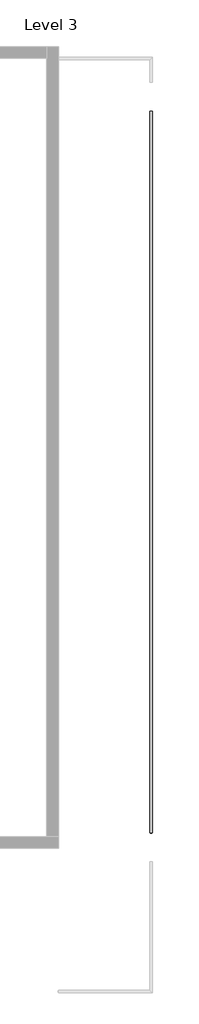
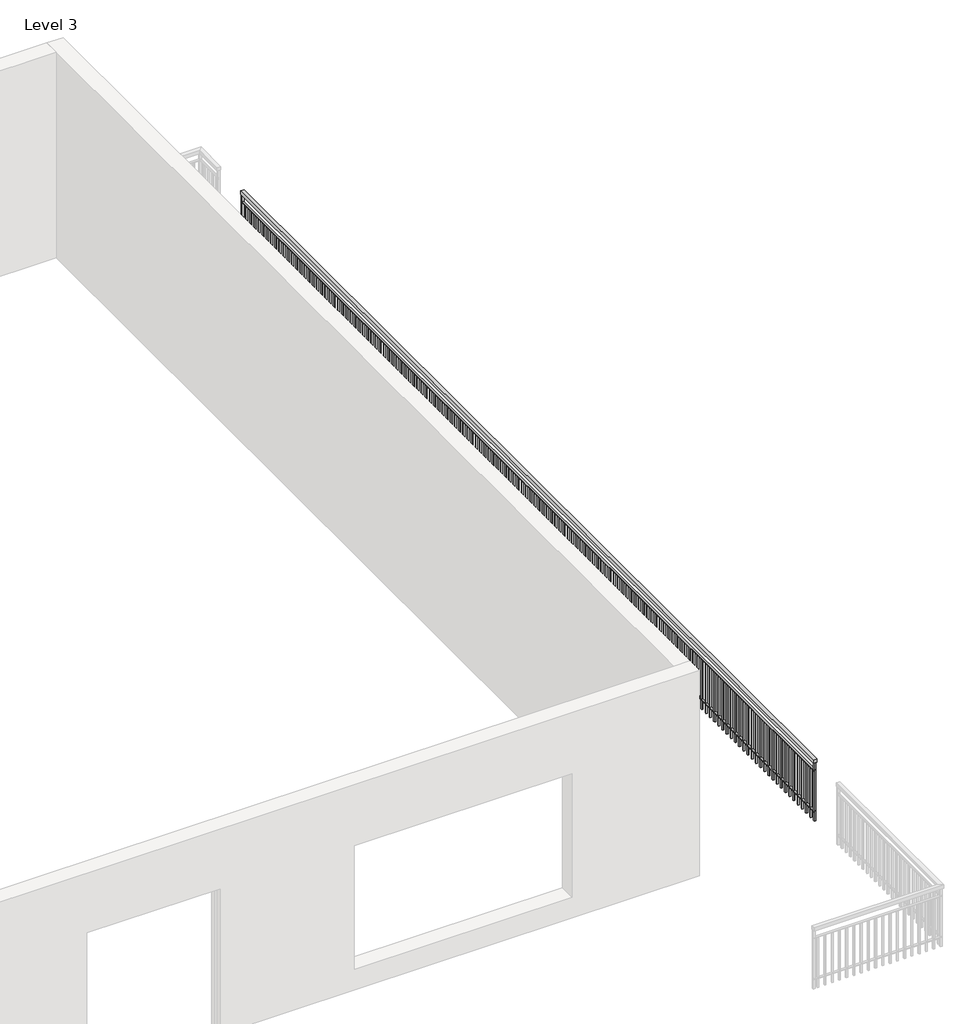
# One storey, part 3 of 4: 1 railing.
"""IFC4 building model written with IfcOpenShell, lengths in millimetres."""

from ifc_helpers import new_model, si_unit, point, frame, frame_2d, origin, place, context, project, spatial, polyline, circle_curve, trimmed, segment, composite_curve, outline, extrude, element, save

model = new_model("IFC4")

# Units and contexts
model_context = context("Model", 3, world=origin())
ifc_project = project(units=[si_unit("LENGTHUNIT", "METRE", prefix="MILLI")], contexts=[model_context])

# Site, building, storey
site = spatial("IfcSite", under=ifc_project)
building = spatial("IfcBuilding", under=site)
storey = spatial("IfcBuildingStorey", under=building, Name="Level 3", Elevation=3810.0)

# Railing
placement = place(None, origin())
element("IfcRailing", 1, ObjectType="Handrail - Rectangular", at=placement, inside=storey, context=model_context, shape_type="SweptSolid", body=[
    extrude(outline(polyline([(8462.6425759, 8145.5475503), (8513.4425759, 8145.5475503), (8513.4425759, -5773.6524497), (8462.6425759, -5773.6524497), (8462.6425759, 8145.5475503)])), frame((0.0, 0.0, 4673.6), z_axis=(0.0, 0.0, 1.0), x_axis=(1.0, 0.0, 0.0)), (0.0, 0.0, 1.0), 50.8),
    extrude(outline(composite_curve([segment(trimmed(circle_curve(frame_2d((4559.3, 8488.0425759)), 12.7), [point((4559.3, 8500.7425759))], [point((4559.3, 8475.3425759))], False, "CARTESIAN"), True, "CONTINUOUS"), segment(trimmed(circle_curve(frame_2d((4559.3, 8488.0425759)), 12.7), [point((4559.3, 8475.3425759))], [point((4559.3, 8500.7425759))], False, "CARTESIAN"), True, "CONTINUOUS")], self_intersect=False)), frame((0.0, -5773.6524497, 0.0), z_axis=(0.0, 1.0, 0.0), x_axis=(0.0, 0.0, 1.0)), (0.0, 0.0, 1.0), 13919.2),
    extrude(outline(composite_curve([segment(trimmed(circle_curve(frame_2d((3949.7, 8488.0425759)), 12.7), [point((3949.7, 8500.7425759))], [point((3949.7, 8475.3425759))], False, "CARTESIAN"), True, "CONTINUOUS"), segment(trimmed(circle_curve(frame_2d((3949.7, 8488.0425759)), 12.7), [point((3949.7, 8475.3425759))], [point((3949.7, 8500.7425759))], False, "CARTESIAN"), True, "CONTINUOUS")], self_intersect=False)), frame((0.0, -5773.6524497, 0.0), z_axis=(0.0, 1.0, 0.0), x_axis=(0.0, 0.0, 1.0)), (0.0, 0.0, 1.0), 13919.2),
    extrude(outline(polyline([(8478.5175759, -5662.5274497), (8497.5675759, -5662.5274497), (8497.5675759, -5681.5774497), (8478.5175759, -5681.5774497), (8478.5175759, -5662.5274497)])), frame((0.0, 0.0, 3810.0), z_axis=(0.0, 0.0, 1.0), x_axis=(1.0, 0.0, 0.0)), (0.0, 0.0, 1.0), 736.6),
    extrude(outline(polyline([(8478.5175759, -5560.9274497), (8497.5675759, -5560.9274497), (8497.5675759, -5579.9774497), (8478.5175759, -5579.9774497), (8478.5175759, -5560.9274497)])), frame((0.0, 0.0, 3810.0), z_axis=(0.0, 0.0, 1.0), x_axis=(1.0, 0.0, 0.0)), (0.0, 0.0, 1.0), 736.6),
    extrude(outline(polyline([(8478.5175759, -5459.3274497), (8497.5675759, -5459.3274497), (8497.5675759, -5478.3774497), (8478.5175759, -5478.3774497), (8478.5175759, -5459.3274497)])), frame((0.0, 0.0, 3810.0), z_axis=(0.0, 0.0, 1.0), x_axis=(1.0, 0.0, 0.0)), (0.0, 0.0, 1.0), 736.6),
    extrude(outline(polyline([(8478.5175759, -5357.7274497), (8497.5675759, -5357.7274497), (8497.5675759, -5376.7774497), (8478.5175759, -5376.7774497), (8478.5175759, -5357.7274497)])), frame((0.0, 0.0, 3810.0), z_axis=(0.0, 0.0, 1.0), x_axis=(1.0, 0.0, 0.0)), (0.0, 0.0, 1.0), 736.6),
    extrude(outline(polyline([(8478.5175759, -5256.1274497), (8497.5675759, -5256.1274497), (8497.5675759, -5275.1774497), (8478.5175759, -5275.1774497), (8478.5175759, -5256.1274497)])), frame((0.0, 0.0, 3810.0), z_axis=(0.0, 0.0, 1.0), x_axis=(1.0, 0.0, 0.0)), (0.0, 0.0, 1.0), 736.6),
    extrude(outline(polyline([(8478.5175759, -5154.5274497), (8497.5675759, -5154.5274497), (8497.5675759, -5173.5774497), (8478.5175759, -5173.5774497), (8478.5175759, -5154.5274497)])), frame((0.0, 0.0, 3810.0), z_axis=(0.0, 0.0, 1.0), x_axis=(1.0, 0.0, 0.0)), (0.0, 0.0, 1.0), 736.6),
    extrude(outline(polyline([(8478.5175759, -5052.9274497), (8497.5675759, -5052.9274497), (8497.5675759, -5071.9774497), (8478.5175759, -5071.9774497), (8478.5175759, -5052.9274497)])), frame((0.0, 0.0, 3810.0), z_axis=(0.0, 0.0, 1.0), x_axis=(1.0, 0.0, 0.0)), (0.0, 0.0, 1.0), 736.6),
    extrude(outline(polyline([(8478.5175759, -4951.3274497), (8497.5675759, -4951.3274497), (8497.5675759, -4970.3774497), (8478.5175759, -4970.3774497), (8478.5175759, -4951.3274497)])), frame((0.0, 0.0, 3810.0), z_axis=(0.0, 0.0, 1.0), x_axis=(1.0, 0.0, 0.0)), (0.0, 0.0, 1.0), 736.6),
    extrude(outline(polyline([(8478.5175759, -4849.7274497), (8497.5675759, -4849.7274497), (8497.5675759, -4868.7774497), (8478.5175759, -4868.7774497), (8478.5175759, -4849.7274497)])), frame((0.0, 0.0, 3810.0), z_axis=(0.0, 0.0, 1.0), x_axis=(1.0, 0.0, 0.0)), (0.0, 0.0, 1.0), 736.6),
    extrude(outline(polyline([(8478.5175759, -4748.1274497), (8497.5675759, -4748.1274497), (8497.5675759, -4767.1774497), (8478.5175759, -4767.1774497), (8478.5175759, -4748.1274497)])), frame((0.0, 0.0, 3810.0), z_axis=(0.0, 0.0, 1.0), x_axis=(1.0, 0.0, 0.0)), (0.0, 0.0, 1.0), 736.6),
    extrude(outline(polyline([(8478.5175759, -4646.5274497), (8497.5675759, -4646.5274497), (8497.5675759, -4665.5774497), (8478.5175759, -4665.5774497), (8478.5175759, -4646.5274497)])), frame((0.0, 0.0, 3810.0), z_axis=(0.0, 0.0, 1.0), x_axis=(1.0, 0.0, 0.0)), (0.0, 0.0, 1.0), 736.6),
    extrude(outline(polyline([(8478.5175759, -4544.9274497), (8497.5675759, -4544.9274497), (8497.5675759, -4563.9774497), (8478.5175759, -4563.9774497), (8478.5175759, -4544.9274497)])), frame((0.0, 0.0, 3810.0), z_axis=(0.0, 0.0, 1.0), x_axis=(1.0, 0.0, 0.0)), (0.0, 0.0, 1.0), 736.6),
    extrude(outline(polyline([(8478.5175759, -4443.3274497), (8497.5675759, -4443.3274497), (8497.5675759, -4462.3774497), (8478.5175759, -4462.3774497), (8478.5175759, -4443.3274497)])), frame((0.0, 0.0, 3810.0), z_axis=(0.0, 0.0, 1.0), x_axis=(1.0, 0.0, 0.0)), (0.0, 0.0, 1.0), 736.6),
    extrude(outline(polyline([(8478.5175759, -4341.7274497), (8497.5675759, -4341.7274497), (8497.5675759, -4360.7774497), (8478.5175759, -4360.7774497), (8478.5175759, -4341.7274497)])), frame((0.0, 0.0, 3810.0), z_axis=(0.0, 0.0, 1.0), x_axis=(1.0, 0.0, 0.0)), (0.0, 0.0, 1.0), 736.6),
    extrude(outline(polyline([(8478.5175759, -4240.1274497), (8497.5675759, -4240.1274497), (8497.5675759, -4259.1774497), (8478.5175759, -4259.1774497), (8478.5175759, -4240.1274497)])), frame((0.0, 0.0, 3810.0), z_axis=(0.0, 0.0, 1.0), x_axis=(1.0, 0.0, 0.0)), (0.0, 0.0, 1.0), 736.6),
    extrude(outline(polyline([(8478.5175759, -4138.5274497), (8497.5675759, -4138.5274497), (8497.5675759, -4157.5774497), (8478.5175759, -4157.5774497), (8478.5175759, -4138.5274497)])), frame((0.0, 0.0, 3810.0), z_axis=(0.0, 0.0, 1.0), x_axis=(1.0, 0.0, 0.0)), (0.0, 0.0, 1.0), 736.6),
    extrude(outline(polyline([(8478.5175759, -4036.9274497), (8497.5675759, -4036.9274497), (8497.5675759, -4055.9774497), (8478.5175759, -4055.9774497), (8478.5175759, -4036.9274497)])), frame((0.0, 0.0, 3810.0), z_axis=(0.0, 0.0, 1.0), x_axis=(1.0, 0.0, 0.0)), (0.0, 0.0, 1.0), 736.6),
    extrude(outline(polyline([(8478.5175759, -3935.3274497), (8497.5675759, -3935.3274497), (8497.5675759, -3954.3774497), (8478.5175759, -3954.3774497), (8478.5175759, -3935.3274497)])), frame((0.0, 0.0, 3810.0), z_axis=(0.0, 0.0, 1.0), x_axis=(1.0, 0.0, 0.0)), (0.0, 0.0, 1.0), 736.6),
    extrude(outline(polyline([(8478.5175759, -3833.7274497), (8497.5675759, -3833.7274497), (8497.5675759, -3852.7774497), (8478.5175759, -3852.7774497), (8478.5175759, -3833.7274497)])), frame((0.0, 0.0, 3810.0), z_axis=(0.0, 0.0, 1.0), x_axis=(1.0, 0.0, 0.0)), (0.0, 0.0, 1.0), 736.6),
    extrude(outline(polyline([(8478.5175759, -3732.1274497), (8497.5675759, -3732.1274497), (8497.5675759, -3751.1774497), (8478.5175759, -3751.1774497), (8478.5175759, -3732.1274497)])), frame((0.0, 0.0, 3810.0), z_axis=(0.0, 0.0, 1.0), x_axis=(1.0, 0.0, 0.0)), (0.0, 0.0, 1.0), 736.6),
    extrude(outline(polyline([(8478.5175759, -3630.5274497), (8497.5675759, -3630.5274497), (8497.5675759, -3649.5774497), (8478.5175759, -3649.5774497), (8478.5175759, -3630.5274497)])), frame((0.0, 0.0, 3810.0), z_axis=(0.0, 0.0, 1.0), x_axis=(1.0, 0.0, 0.0)), (0.0, 0.0, 1.0), 736.6),
    extrude(outline(polyline([(8478.5175759, -3528.9274497), (8497.5675759, -3528.9274497), (8497.5675759, -3547.9774497), (8478.5175759, -3547.9774497), (8478.5175759, -3528.9274497)])), frame((0.0, 0.0, 3810.0), z_axis=(0.0, 0.0, 1.0), x_axis=(1.0, 0.0, 0.0)), (0.0, 0.0, 1.0), 736.6),
    extrude(outline(polyline([(8478.5175759, -3427.3274497), (8497.5675759, -3427.3274497), (8497.5675759, -3446.3774497), (8478.5175759, -3446.3774497), (8478.5175759, -3427.3274497)])), frame((0.0, 0.0, 3810.0), z_axis=(0.0, 0.0, 1.0), x_axis=(1.0, 0.0, 0.0)), (0.0, 0.0, 1.0), 736.6),
    extrude(outline(polyline([(8478.5175759, -3325.7274497), (8497.5675759, -3325.7274497), (8497.5675759, -3344.7774497), (8478.5175759, -3344.7774497), (8478.5175759, -3325.7274497)])), frame((0.0, 0.0, 3810.0), z_axis=(0.0, 0.0, 1.0), x_axis=(1.0, 0.0, 0.0)), (0.0, 0.0, 1.0), 736.6),
    extrude(outline(polyline([(8478.5175759, -3224.1274497), (8497.5675759, -3224.1274497), (8497.5675759, -3243.1774497), (8478.5175759, -3243.1774497), (8478.5175759, -3224.1274497)])), frame((0.0, 0.0, 3810.0), z_axis=(0.0, 0.0, 1.0), x_axis=(1.0, 0.0, 0.0)), (0.0, 0.0, 1.0), 736.6),
    extrude(outline(polyline([(8478.5175759, -3122.5274497), (8497.5675759, -3122.5274497), (8497.5675759, -3141.5774497), (8478.5175759, -3141.5774497), (8478.5175759, -3122.5274497)])), frame((0.0, 0.0, 3810.0), z_axis=(0.0, 0.0, 1.0), x_axis=(1.0, 0.0, 0.0)), (0.0, 0.0, 1.0), 736.6),
    extrude(outline(polyline([(8478.5175759, -3020.9274497), (8497.5675759, -3020.9274497), (8497.5675759, -3039.9774497), (8478.5175759, -3039.9774497), (8478.5175759, -3020.9274497)])), frame((0.0, 0.0, 3810.0), z_axis=(0.0, 0.0, 1.0), x_axis=(1.0, 0.0, 0.0)), (0.0, 0.0, 1.0), 736.6),
    extrude(outline(polyline([(8478.5175759, -2919.3274497), (8497.5675759, -2919.3274497), (8497.5675759, -2938.3774497), (8478.5175759, -2938.3774497), (8478.5175759, -2919.3274497)])), frame((0.0, 0.0, 3810.0), z_axis=(0.0, 0.0, 1.0), x_axis=(1.0, 0.0, 0.0)), (0.0, 0.0, 1.0), 736.6),
    extrude(outline(polyline([(8478.5175759, -2817.7274497), (8497.5675759, -2817.7274497), (8497.5675759, -2836.7774497), (8478.5175759, -2836.7774497), (8478.5175759, -2817.7274497)])), frame((0.0, 0.0, 3810.0), z_axis=(0.0, 0.0, 1.0), x_axis=(1.0, 0.0, 0.0)), (0.0, 0.0, 1.0), 736.6),
    extrude(outline(polyline([(8478.5175759, -2716.1274497), (8497.5675759, -2716.1274497), (8497.5675759, -2735.1774497), (8478.5175759, -2735.1774497), (8478.5175759, -2716.1274497)])), frame((0.0, 0.0, 3810.0), z_axis=(0.0, 0.0, 1.0), x_axis=(1.0, 0.0, 0.0)), (0.0, 0.0, 1.0), 736.6),
    extrude(outline(polyline([(8478.5175759, -2614.5274497), (8497.5675759, -2614.5274497), (8497.5675759, -2633.5774497), (8478.5175759, -2633.5774497), (8478.5175759, -2614.5274497)])), frame((0.0, 0.0, 3810.0), z_axis=(0.0, 0.0, 1.0), x_axis=(1.0, 0.0, 0.0)), (0.0, 0.0, 1.0), 736.6),
    extrude(outline(polyline([(8478.5175759, -2512.9274497), (8497.5675759, -2512.9274497), (8497.5675759, -2531.9774497), (8478.5175759, -2531.9774497), (8478.5175759, -2512.9274497)])), frame((0.0, 0.0, 3810.0), z_axis=(0.0, 0.0, 1.0), x_axis=(1.0, 0.0, 0.0)), (0.0, 0.0, 1.0), 736.6),
    extrude(outline(polyline([(8478.5175759, -2411.3274497), (8497.5675759, -2411.3274497), (8497.5675759, -2430.3774497), (8478.5175759, -2430.3774497), (8478.5175759, -2411.3274497)])), frame((0.0, 0.0, 3810.0), z_axis=(0.0, 0.0, 1.0), x_axis=(1.0, 0.0, 0.0)), (0.0, 0.0, 1.0), 736.6),
    extrude(outline(polyline([(8478.5175759, -2309.7274497), (8497.5675759, -2309.7274497), (8497.5675759, -2328.7774497), (8478.5175759, -2328.7774497), (8478.5175759, -2309.7274497)])), frame((0.0, 0.0, 3810.0), z_axis=(0.0, 0.0, 1.0), x_axis=(1.0, 0.0, 0.0)), (0.0, 0.0, 1.0), 736.6),
    extrude(outline(polyline([(8478.5175759, -2208.1274497), (8497.5675759, -2208.1274497), (8497.5675759, -2227.1774497), (8478.5175759, -2227.1774497), (8478.5175759, -2208.1274497)])), frame((0.0, 0.0, 3810.0), z_axis=(0.0, 0.0, 1.0), x_axis=(1.0, 0.0, 0.0)), (0.0, 0.0, 1.0), 736.6),
    extrude(outline(polyline([(8478.5175759, -2106.5274497), (8497.5675759, -2106.5274497), (8497.5675759, -2125.5774497), (8478.5175759, -2125.5774497), (8478.5175759, -2106.5274497)])), frame((0.0, 0.0, 3810.0), z_axis=(0.0, 0.0, 1.0), x_axis=(1.0, 0.0, 0.0)), (0.0, 0.0, 1.0), 736.6),
    extrude(outline(polyline([(8478.5175759, -2004.9274497), (8497.5675759, -2004.9274497), (8497.5675759, -2023.9774497), (8478.5175759, -2023.9774497), (8478.5175759, -2004.9274497)])), frame((0.0, 0.0, 3810.0), z_axis=(0.0, 0.0, 1.0), x_axis=(1.0, 0.0, 0.0)), (0.0, 0.0, 1.0), 736.6),
    extrude(outline(polyline([(8478.5175759, -1903.3274497), (8497.5675759, -1903.3274497), (8497.5675759, -1922.3774497), (8478.5175759, -1922.3774497), (8478.5175759, -1903.3274497)])), frame((0.0, 0.0, 3810.0), z_axis=(0.0, 0.0, 1.0), x_axis=(1.0, 0.0, 0.0)), (0.0, 0.0, 1.0), 736.6),
    extrude(outline(polyline([(8478.5175759, -1801.7274497), (8497.5675759, -1801.7274497), (8497.5675759, -1820.7774497), (8478.5175759, -1820.7774497), (8478.5175759, -1801.7274497)])), frame((0.0, 0.0, 3810.0), z_axis=(0.0, 0.0, 1.0), x_axis=(1.0, 0.0, 0.0)), (0.0, 0.0, 1.0), 736.6),
    extrude(outline(polyline([(8478.5175759, -1700.1274497), (8497.5675759, -1700.1274497), (8497.5675759, -1719.1774497), (8478.5175759, -1719.1774497), (8478.5175759, -1700.1274497)])), frame((0.0, 0.0, 3810.0), z_axis=(0.0, 0.0, 1.0), x_axis=(1.0, 0.0, 0.0)), (0.0, 0.0, 1.0), 736.6),
    extrude(outline(polyline([(8478.5175759, -1598.5274497), (8497.5675759, -1598.5274497), (8497.5675759, -1617.5774497), (8478.5175759, -1617.5774497), (8478.5175759, -1598.5274497)])), frame((0.0, 0.0, 3810.0), z_axis=(0.0, 0.0, 1.0), x_axis=(1.0, 0.0, 0.0)), (0.0, 0.0, 1.0), 736.6),
    extrude(outline(polyline([(8478.5175759, -1496.9274497), (8497.5675759, -1496.9274497), (8497.5675759, -1515.9774497), (8478.5175759, -1515.9774497), (8478.5175759, -1496.9274497)])), frame((0.0, 0.0, 3810.0), z_axis=(0.0, 0.0, 1.0), x_axis=(1.0, 0.0, 0.0)), (0.0, 0.0, 1.0), 736.6),
    extrude(outline(polyline([(8478.5175759, -1395.3274497), (8497.5675759, -1395.3274497), (8497.5675759, -1414.3774497), (8478.5175759, -1414.3774497), (8478.5175759, -1395.3274497)])), frame((0.0, 0.0, 3810.0), z_axis=(0.0, 0.0, 1.0), x_axis=(1.0, 0.0, 0.0)), (0.0, 0.0, 1.0), 736.6),
    extrude(outline(polyline([(8478.5175759, -1293.7274497), (8497.5675759, -1293.7274497), (8497.5675759, -1312.7774497), (8478.5175759, -1312.7774497), (8478.5175759, -1293.7274497)])), frame((0.0, 0.0, 3810.0), z_axis=(0.0, 0.0, 1.0), x_axis=(1.0, 0.0, 0.0)), (0.0, 0.0, 1.0), 736.6),
    extrude(outline(polyline([(8478.5175759, -1192.1274497), (8497.5675759, -1192.1274497), (8497.5675759, -1211.1774497), (8478.5175759, -1211.1774497), (8478.5175759, -1192.1274497)])), frame((0.0, 0.0, 3810.0), z_axis=(0.0, 0.0, 1.0), x_axis=(1.0, 0.0, 0.0)), (0.0, 0.0, 1.0), 736.6),
    extrude(outline(polyline([(8478.5175759, -1090.5274497), (8497.5675759, -1090.5274497), (8497.5675759, -1109.5774497), (8478.5175759, -1109.5774497), (8478.5175759, -1090.5274497)])), frame((0.0, 0.0, 3810.0), z_axis=(0.0, 0.0, 1.0), x_axis=(1.0, 0.0, 0.0)), (0.0, 0.0, 1.0), 736.6),
    extrude(outline(polyline([(8478.5175759, -988.9274497), (8497.5675759, -988.9274497), (8497.5675759, -1007.9774497), (8478.5175759, -1007.9774497), (8478.5175759, -988.9274497)])), frame((0.0, 0.0, 3810.0), z_axis=(0.0, 0.0, 1.0), x_axis=(1.0, 0.0, 0.0)), (0.0, 0.0, 1.0), 736.6),
    extrude(outline(polyline([(8478.5175759, -887.3274497), (8497.5675759, -887.3274497), (8497.5675759, -906.3774497), (8478.5175759, -906.3774497), (8478.5175759, -887.3274497)])), frame((0.0, 0.0, 3810.0), z_axis=(0.0, 0.0, 1.0), x_axis=(1.0, 0.0, 0.0)), (0.0, 0.0, 1.0), 736.6),
    extrude(outline(polyline([(8478.5175759, -785.7274497), (8497.5675759, -785.7274497), (8497.5675759, -804.7774497), (8478.5175759, -804.7774497), (8478.5175759, -785.7274497)])), frame((0.0, 0.0, 3810.0), z_axis=(0.0, 0.0, 1.0), x_axis=(1.0, 0.0, 0.0)), (0.0, 0.0, 1.0), 736.6),
    extrude(outline(polyline([(8478.5175759, -684.1274497), (8497.5675759, -684.1274497), (8497.5675759, -703.1774497), (8478.5175759, -703.1774497), (8478.5175759, -684.1274497)])), frame((0.0, 0.0, 3810.0), z_axis=(0.0, 0.0, 1.0), x_axis=(1.0, 0.0, 0.0)), (0.0, 0.0, 1.0), 736.6),
    extrude(outline(polyline([(8478.5175759, -582.5274497), (8497.5675759, -582.5274497), (8497.5675759, -601.5774497), (8478.5175759, -601.5774497), (8478.5175759, -582.5274497)])), frame((0.0, 0.0, 3810.0), z_axis=(0.0, 0.0, 1.0), x_axis=(1.0, 0.0, 0.0)), (0.0, 0.0, 1.0), 736.6),
    extrude(outline(polyline([(8478.5175759, -480.9274497), (8497.5675759, -480.9274497), (8497.5675759, -499.9774497), (8478.5175759, -499.9774497), (8478.5175759, -480.9274497)])), frame((0.0, 0.0, 3810.0), z_axis=(0.0, 0.0, 1.0), x_axis=(1.0, 0.0, 0.0)), (0.0, 0.0, 1.0), 736.6),
    extrude(outline(polyline([(8478.5175759, -379.3274497), (8497.5675759, -379.3274497), (8497.5675759, -398.3774497), (8478.5175759, -398.3774497), (8478.5175759, -379.3274497)])), frame((0.0, 0.0, 3810.0), z_axis=(0.0, 0.0, 1.0), x_axis=(1.0, 0.0, 0.0)), (0.0, 0.0, 1.0), 736.6),
    extrude(outline(polyline([(8478.5175759, -277.7274497), (8497.5675759, -277.7274497), (8497.5675759, -296.7774497), (8478.5175759, -296.7774497), (8478.5175759, -277.7274497)])), frame((0.0, 0.0, 3810.0), z_axis=(0.0, 0.0, 1.0), x_axis=(1.0, 0.0, 0.0)), (0.0, 0.0, 1.0), 736.6),
    extrude(outline(polyline([(8478.5175759, -176.1274497), (8497.5675759, -176.1274497), (8497.5675759, -195.1774497), (8478.5175759, -195.1774497), (8478.5175759, -176.1274497)])), frame((0.0, 0.0, 3810.0), z_axis=(0.0, 0.0, 1.0), x_axis=(1.0, 0.0, 0.0)), (0.0, 0.0, 1.0), 736.6),
    extrude(outline(polyline([(8478.5175759, -74.5274497), (8497.5675759, -74.5274497), (8497.5675759, -93.5774497), (8478.5175759, -93.5774497), (8478.5175759, -74.5274497)])), frame((0.0, 0.0, 3810.0), z_axis=(0.0, 0.0, 1.0), x_axis=(1.0, 0.0, 0.0)), (0.0, 0.0, 1.0), 736.6),
    extrude(outline(polyline([(8478.5175759, 27.0725503), (8497.5675759, 27.0725503), (8497.5675759, 8.0225503), (8478.5175759, 8.0225503), (8478.5175759, 27.0725503)])), frame((0.0, 0.0, 3810.0), z_axis=(0.0, 0.0, 1.0), x_axis=(1.0, 0.0, 0.0)), (0.0, 0.0, 1.0), 736.6),
    extrude(outline(polyline([(8478.5175759, 128.6725503), (8497.5675759, 128.6725503), (8497.5675759, 109.6225503), (8478.5175759, 109.6225503), (8478.5175759, 128.6725503)])), frame((0.0, 0.0, 3810.0), z_axis=(0.0, 0.0, 1.0), x_axis=(1.0, 0.0, 0.0)), (0.0, 0.0, 1.0), 736.6),
    extrude(outline(polyline([(8478.5175759, 230.2725503), (8497.5675759, 230.2725503), (8497.5675759, 211.2225503), (8478.5175759, 211.2225503), (8478.5175759, 230.2725503)])), frame((0.0, 0.0, 3810.0), z_axis=(0.0, 0.0, 1.0), x_axis=(1.0, 0.0, 0.0)), (0.0, 0.0, 1.0), 736.6),
    extrude(outline(polyline([(8478.5175759, 331.8725503), (8497.5675759, 331.8725503), (8497.5675759, 312.8225503), (8478.5175759, 312.8225503), (8478.5175759, 331.8725503)])), frame((0.0, 0.0, 3810.0), z_axis=(0.0, 0.0, 1.0), x_axis=(1.0, 0.0, 0.0)), (0.0, 0.0, 1.0), 736.6),
    extrude(outline(polyline([(8478.5175759, 433.4725503), (8497.5675759, 433.4725503), (8497.5675759, 414.4225503), (8478.5175759, 414.4225503), (8478.5175759, 433.4725503)])), frame((0.0, 0.0, 3810.0), z_axis=(0.0, 0.0, 1.0), x_axis=(1.0, 0.0, 0.0)), (0.0, 0.0, 1.0), 736.6),
    extrude(outline(polyline([(8478.5175759, 535.0725503), (8497.5675759, 535.0725503), (8497.5675759, 516.0225503), (8478.5175759, 516.0225503), (8478.5175759, 535.0725503)])), frame((0.0, 0.0, 3810.0), z_axis=(0.0, 0.0, 1.0), x_axis=(1.0, 0.0, 0.0)), (0.0, 0.0, 1.0), 736.6),
    extrude(outline(polyline([(8478.5175759, 636.6725503), (8497.5675759, 636.6725503), (8497.5675759, 617.6225503), (8478.5175759, 617.6225503), (8478.5175759, 636.6725503)])), frame((0.0, 0.0, 3810.0), z_axis=(0.0, 0.0, 1.0), x_axis=(1.0, 0.0, 0.0)), (0.0, 0.0, 1.0), 736.6),
    extrude(outline(polyline([(8478.5175759, 738.2725503), (8497.5675759, 738.2725503), (8497.5675759, 719.2225503), (8478.5175759, 719.2225503), (8478.5175759, 738.2725503)])), frame((0.0, 0.0, 3810.0), z_axis=(0.0, 0.0, 1.0), x_axis=(1.0, 0.0, 0.0)), (0.0, 0.0, 1.0), 736.6),
    extrude(outline(polyline([(8478.5175759, 839.8725503), (8497.5675759, 839.8725503), (8497.5675759, 820.8225503), (8478.5175759, 820.8225503), (8478.5175759, 839.8725503)])), frame((0.0, 0.0, 3810.0), z_axis=(0.0, 0.0, 1.0), x_axis=(1.0, 0.0, 0.0)), (0.0, 0.0, 1.0), 736.6),
    extrude(outline(polyline([(8478.5175759, 941.4725503), (8497.5675759, 941.4725503), (8497.5675759, 922.4225503), (8478.5175759, 922.4225503), (8478.5175759, 941.4725503)])), frame((0.0, 0.0, 3810.0), z_axis=(0.0, 0.0, 1.0), x_axis=(1.0, 0.0, 0.0)), (0.0, 0.0, 1.0), 736.6),
    extrude(outline(polyline([(8478.5175759, 1043.0725503), (8497.5675759, 1043.0725503), (8497.5675759, 1024.0225503), (8478.5175759, 1024.0225503), (8478.5175759, 1043.0725503)])), frame((0.0, 0.0, 3810.0), z_axis=(0.0, 0.0, 1.0), x_axis=(1.0, 0.0, 0.0)), (0.0, 0.0, 1.0), 736.6),
    extrude(outline(polyline([(8478.5175759, 1144.6725503), (8497.5675759, 1144.6725503), (8497.5675759, 1125.6225503), (8478.5175759, 1125.6225503), (8478.5175759, 1144.6725503)])), frame((0.0, 0.0, 3810.0), z_axis=(0.0, 0.0, 1.0), x_axis=(1.0, 0.0, 0.0)), (0.0, 0.0, 1.0), 736.6),
    extrude(outline(polyline([(8478.5175759, 1246.2725503), (8497.5675759, 1246.2725503), (8497.5675759, 1227.2225503), (8478.5175759, 1227.2225503), (8478.5175759, 1246.2725503)])), frame((0.0, 0.0, 3810.0), z_axis=(0.0, 0.0, 1.0), x_axis=(1.0, 0.0, 0.0)), (0.0, 0.0, 1.0), 736.6),
    extrude(outline(polyline([(8478.5175759, 1347.8725503), (8497.5675759, 1347.8725503), (8497.5675759, 1328.8225503), (8478.5175759, 1328.8225503), (8478.5175759, 1347.8725503)])), frame((0.0, 0.0, 3810.0), z_axis=(0.0, 0.0, 1.0), x_axis=(1.0, 0.0, 0.0)), (0.0, 0.0, 1.0), 736.6),
    extrude(outline(polyline([(8478.5175759, 1449.4725503), (8497.5675759, 1449.4725503), (8497.5675759, 1430.4225503), (8478.5175759, 1430.4225503), (8478.5175759, 1449.4725503)])), frame((0.0, 0.0, 3810.0), z_axis=(0.0, 0.0, 1.0), x_axis=(1.0, 0.0, 0.0)), (0.0, 0.0, 1.0), 736.6),
    extrude(outline(polyline([(8478.5175759, 1551.0725503), (8497.5675759, 1551.0725503), (8497.5675759, 1532.0225503), (8478.5175759, 1532.0225503), (8478.5175759, 1551.0725503)])), frame((0.0, 0.0, 3810.0), z_axis=(0.0, 0.0, 1.0), x_axis=(1.0, 0.0, 0.0)), (0.0, 0.0, 1.0), 736.6),
    extrude(outline(polyline([(8478.5175759, 1652.6725503), (8497.5675759, 1652.6725503), (8497.5675759, 1633.6225503), (8478.5175759, 1633.6225503), (8478.5175759, 1652.6725503)])), frame((0.0, 0.0, 3810.0), z_axis=(0.0, 0.0, 1.0), x_axis=(1.0, 0.0, 0.0)), (0.0, 0.0, 1.0), 736.6),
    extrude(outline(polyline([(8478.5175759, 1754.2725503), (8497.5675759, 1754.2725503), (8497.5675759, 1735.2225503), (8478.5175759, 1735.2225503), (8478.5175759, 1754.2725503)])), frame((0.0, 0.0, 3810.0), z_axis=(0.0, 0.0, 1.0), x_axis=(1.0, 0.0, 0.0)), (0.0, 0.0, 1.0), 736.6),
    extrude(outline(polyline([(8478.5175759, 1855.8725503), (8497.5675759, 1855.8725503), (8497.5675759, 1836.8225503), (8478.5175759, 1836.8225503), (8478.5175759, 1855.8725503)])), frame((0.0, 0.0, 3810.0), z_axis=(0.0, 0.0, 1.0), x_axis=(1.0, 0.0, 0.0)), (0.0, 0.0, 1.0), 736.6),
    extrude(outline(polyline([(8478.5175759, 1957.4725503), (8497.5675759, 1957.4725503), (8497.5675759, 1938.4225503), (8478.5175759, 1938.4225503), (8478.5175759, 1957.4725503)])), frame((0.0, 0.0, 3810.0), z_axis=(0.0, 0.0, 1.0), x_axis=(1.0, 0.0, 0.0)), (0.0, 0.0, 1.0), 736.6),
    extrude(outline(polyline([(8478.5175759, 2059.0725503), (8497.5675759, 2059.0725503), (8497.5675759, 2040.0225503), (8478.5175759, 2040.0225503), (8478.5175759, 2059.0725503)])), frame((0.0, 0.0, 3810.0), z_axis=(0.0, 0.0, 1.0), x_axis=(1.0, 0.0, 0.0)), (0.0, 0.0, 1.0), 736.6),
    extrude(outline(polyline([(8478.5175759, 2160.6725503), (8497.5675759, 2160.6725503), (8497.5675759, 2141.6225503), (8478.5175759, 2141.6225503), (8478.5175759, 2160.6725503)])), frame((0.0, 0.0, 3810.0), z_axis=(0.0, 0.0, 1.0), x_axis=(1.0, 0.0, 0.0)), (0.0, 0.0, 1.0), 736.6),
    extrude(outline(polyline([(8478.5175759, 2262.2725503), (8497.5675759, 2262.2725503), (8497.5675759, 2243.2225503), (8478.5175759, 2243.2225503), (8478.5175759, 2262.2725503)])), frame((0.0, 0.0, 3810.0), z_axis=(0.0, 0.0, 1.0), x_axis=(1.0, 0.0, 0.0)), (0.0, 0.0, 1.0), 736.6),
    extrude(outline(polyline([(8478.5175759, 2363.8725503), (8497.5675759, 2363.8725503), (8497.5675759, 2344.8225503), (8478.5175759, 2344.8225503), (8478.5175759, 2363.8725503)])), frame((0.0, 0.0, 3810.0), z_axis=(0.0, 0.0, 1.0), x_axis=(1.0, 0.0, 0.0)), (0.0, 0.0, 1.0), 736.6),
    extrude(outline(polyline([(8478.5175759, 2465.4725503), (8497.5675759, 2465.4725503), (8497.5675759, 2446.4225503), (8478.5175759, 2446.4225503), (8478.5175759, 2465.4725503)])), frame((0.0, 0.0, 3810.0), z_axis=(0.0, 0.0, 1.0), x_axis=(1.0, 0.0, 0.0)), (0.0, 0.0, 1.0), 736.6),
    extrude(outline(polyline([(8478.5175759, 2567.0725503), (8497.5675759, 2567.0725503), (8497.5675759, 2548.0225503), (8478.5175759, 2548.0225503), (8478.5175759, 2567.0725503)])), frame((0.0, 0.0, 3810.0), z_axis=(0.0, 0.0, 1.0), x_axis=(1.0, 0.0, 0.0)), (0.0, 0.0, 1.0), 736.6),
    extrude(outline(polyline([(8478.5175759, 2668.6725503), (8497.5675759, 2668.6725503), (8497.5675759, 2649.6225503), (8478.5175759, 2649.6225503), (8478.5175759, 2668.6725503)])), frame((0.0, 0.0, 3810.0), z_axis=(0.0, 0.0, 1.0), x_axis=(1.0, 0.0, 0.0)), (0.0, 0.0, 1.0), 736.6),
    extrude(outline(polyline([(8478.5175759, 2770.2725503), (8497.5675759, 2770.2725503), (8497.5675759, 2751.2225503), (8478.5175759, 2751.2225503), (8478.5175759, 2770.2725503)])), frame((0.0, 0.0, 3810.0), z_axis=(0.0, 0.0, 1.0), x_axis=(1.0, 0.0, 0.0)), (0.0, 0.0, 1.0), 736.6),
    extrude(outline(polyline([(8478.5175759, 2871.8725503), (8497.5675759, 2871.8725503), (8497.5675759, 2852.8225503), (8478.5175759, 2852.8225503), (8478.5175759, 2871.8725503)])), frame((0.0, 0.0, 3810.0), z_axis=(0.0, 0.0, 1.0), x_axis=(1.0, 0.0, 0.0)), (0.0, 0.0, 1.0), 736.6),
    extrude(outline(polyline([(8478.5175759, 2973.4725503), (8497.5675759, 2973.4725503), (8497.5675759, 2954.4225503), (8478.5175759, 2954.4225503), (8478.5175759, 2973.4725503)])), frame((0.0, 0.0, 3810.0), z_axis=(0.0, 0.0, 1.0), x_axis=(1.0, 0.0, 0.0)), (0.0, 0.0, 1.0), 736.6),
    extrude(outline(polyline([(8478.5175759, 3075.0725503), (8497.5675759, 3075.0725503), (8497.5675759, 3056.0225503), (8478.5175759, 3056.0225503), (8478.5175759, 3075.0725503)])), frame((0.0, 0.0, 3810.0), z_axis=(0.0, 0.0, 1.0), x_axis=(1.0, 0.0, 0.0)), (0.0, 0.0, 1.0), 736.6),
    extrude(outline(polyline([(8478.5175759, 3176.6725503), (8497.5675759, 3176.6725503), (8497.5675759, 3157.6225503), (8478.5175759, 3157.6225503), (8478.5175759, 3176.6725503)])), frame((0.0, 0.0, 3810.0), z_axis=(0.0, 0.0, 1.0), x_axis=(1.0, 0.0, 0.0)), (0.0, 0.0, 1.0), 736.6),
    extrude(outline(polyline([(8478.5175759, 3278.2725503), (8497.5675759, 3278.2725503), (8497.5675759, 3259.2225503), (8478.5175759, 3259.2225503), (8478.5175759, 3278.2725503)])), frame((0.0, 0.0, 3810.0), z_axis=(0.0, 0.0, 1.0), x_axis=(1.0, 0.0, 0.0)), (0.0, 0.0, 1.0), 736.6),
    extrude(outline(polyline([(8478.5175759, 3379.8725503), (8497.5675759, 3379.8725503), (8497.5675759, 3360.8225503), (8478.5175759, 3360.8225503), (8478.5175759, 3379.8725503)])), frame((0.0, 0.0, 3810.0), z_axis=(0.0, 0.0, 1.0), x_axis=(1.0, 0.0, 0.0)), (0.0, 0.0, 1.0), 736.6),
    extrude(outline(polyline([(8478.5175759, 3481.4725503), (8497.5675759, 3481.4725503), (8497.5675759, 3462.4225503), (8478.5175759, 3462.4225503), (8478.5175759, 3481.4725503)])), frame((0.0, 0.0, 3810.0), z_axis=(0.0, 0.0, 1.0), x_axis=(1.0, 0.0, 0.0)), (0.0, 0.0, 1.0), 736.6),
    extrude(outline(polyline([(8478.5175759, 3583.0725503), (8497.5675759, 3583.0725503), (8497.5675759, 3564.0225503), (8478.5175759, 3564.0225503), (8478.5175759, 3583.0725503)])), frame((0.0, 0.0, 3810.0), z_axis=(0.0, 0.0, 1.0), x_axis=(1.0, 0.0, 0.0)), (0.0, 0.0, 1.0), 736.6),
    extrude(outline(polyline([(8478.5175759, 3684.6725503), (8497.5675759, 3684.6725503), (8497.5675759, 3665.6225503), (8478.5175759, 3665.6225503), (8478.5175759, 3684.6725503)])), frame((0.0, 0.0, 3810.0), z_axis=(0.0, 0.0, 1.0), x_axis=(1.0, 0.0, 0.0)), (0.0, 0.0, 1.0), 736.6),
    extrude(outline(polyline([(8478.5175759, 3786.2725503), (8497.5675759, 3786.2725503), (8497.5675759, 3767.2225503), (8478.5175759, 3767.2225503), (8478.5175759, 3786.2725503)])), frame((0.0, 0.0, 3810.0), z_axis=(0.0, 0.0, 1.0), x_axis=(1.0, 0.0, 0.0)), (0.0, 0.0, 1.0), 736.6),
    extrude(outline(polyline([(8478.5175759, 3887.8725503), (8497.5675759, 3887.8725503), (8497.5675759, 3868.8225503), (8478.5175759, 3868.8225503), (8478.5175759, 3887.8725503)])), frame((0.0, 0.0, 3810.0), z_axis=(0.0, 0.0, 1.0), x_axis=(1.0, 0.0, 0.0)), (0.0, 0.0, 1.0), 736.6),
    extrude(outline(polyline([(8478.5175759, 3989.4725503), (8497.5675759, 3989.4725503), (8497.5675759, 3970.4225503), (8478.5175759, 3970.4225503), (8478.5175759, 3989.4725503)])), frame((0.0, 0.0, 3810.0), z_axis=(0.0, 0.0, 1.0), x_axis=(1.0, 0.0, 0.0)), (0.0, 0.0, 1.0), 736.6),
    extrude(outline(polyline([(8478.5175759, 4091.0725503), (8497.5675759, 4091.0725503), (8497.5675759, 4072.0225503), (8478.5175759, 4072.0225503), (8478.5175759, 4091.0725503)])), frame((0.0, 0.0, 3810.0), z_axis=(0.0, 0.0, 1.0), x_axis=(1.0, 0.0, 0.0)), (0.0, 0.0, 1.0), 736.6),
    extrude(outline(polyline([(8478.5175759, 4192.6725503), (8497.5675759, 4192.6725503), (8497.5675759, 4173.6225503), (8478.5175759, 4173.6225503), (8478.5175759, 4192.6725503)])), frame((0.0, 0.0, 3810.0), z_axis=(0.0, 0.0, 1.0), x_axis=(1.0, 0.0, 0.0)), (0.0, 0.0, 1.0), 736.6),
    extrude(outline(polyline([(8478.5175759, 4294.2725503), (8497.5675759, 4294.2725503), (8497.5675759, 4275.2225503), (8478.5175759, 4275.2225503), (8478.5175759, 4294.2725503)])), frame((0.0, 0.0, 3810.0), z_axis=(0.0, 0.0, 1.0), x_axis=(1.0, 0.0, 0.0)), (0.0, 0.0, 1.0), 736.6),
    extrude(outline(polyline([(8478.5175759, 4395.8725503), (8497.5675759, 4395.8725503), (8497.5675759, 4376.8225503), (8478.5175759, 4376.8225503), (8478.5175759, 4395.8725503)])), frame((0.0, 0.0, 3810.0), z_axis=(0.0, 0.0, 1.0), x_axis=(1.0, 0.0, 0.0)), (0.0, 0.0, 1.0), 736.6),
    extrude(outline(polyline([(8478.5175759, 4497.4725503), (8497.5675759, 4497.4725503), (8497.5675759, 4478.4225503), (8478.5175759, 4478.4225503), (8478.5175759, 4497.4725503)])), frame((0.0, 0.0, 3810.0), z_axis=(0.0, 0.0, 1.0), x_axis=(1.0, 0.0, 0.0)), (0.0, 0.0, 1.0), 736.6),
    extrude(outline(polyline([(8478.5175759, 4599.0725503), (8497.5675759, 4599.0725503), (8497.5675759, 4580.0225503), (8478.5175759, 4580.0225503), (8478.5175759, 4599.0725503)])), frame((0.0, 0.0, 3810.0), z_axis=(0.0, 0.0, 1.0), x_axis=(1.0, 0.0, 0.0)), (0.0, 0.0, 1.0), 736.6),
    extrude(outline(polyline([(8478.5175759, 4700.6725503), (8497.5675759, 4700.6725503), (8497.5675759, 4681.6225503), (8478.5175759, 4681.6225503), (8478.5175759, 4700.6725503)])), frame((0.0, 0.0, 3810.0), z_axis=(0.0, 0.0, 1.0), x_axis=(1.0, 0.0, 0.0)), (0.0, 0.0, 1.0), 736.6),
    extrude(outline(polyline([(8478.5175759, 4802.2725503), (8497.5675759, 4802.2725503), (8497.5675759, 4783.2225503), (8478.5175759, 4783.2225503), (8478.5175759, 4802.2725503)])), frame((0.0, 0.0, 3810.0), z_axis=(0.0, 0.0, 1.0), x_axis=(1.0, 0.0, 0.0)), (0.0, 0.0, 1.0), 736.6),
    extrude(outline(polyline([(8478.5175759, 4903.8725503), (8497.5675759, 4903.8725503), (8497.5675759, 4884.8225503), (8478.5175759, 4884.8225503), (8478.5175759, 4903.8725503)])), frame((0.0, 0.0, 3810.0), z_axis=(0.0, 0.0, 1.0), x_axis=(1.0, 0.0, 0.0)), (0.0, 0.0, 1.0), 736.6),
    extrude(outline(polyline([(8478.5175759, 5005.4725503), (8497.5675759, 5005.4725503), (8497.5675759, 4986.4225503), (8478.5175759, 4986.4225503), (8478.5175759, 5005.4725503)])), frame((0.0, 0.0, 3810.0), z_axis=(0.0, 0.0, 1.0), x_axis=(1.0, 0.0, 0.0)), (0.0, 0.0, 1.0), 736.6),
    extrude(outline(polyline([(8478.5175759, 5107.0725503), (8497.5675759, 5107.0725503), (8497.5675759, 5088.0225503), (8478.5175759, 5088.0225503), (8478.5175759, 5107.0725503)])), frame((0.0, 0.0, 3810.0), z_axis=(0.0, 0.0, 1.0), x_axis=(1.0, 0.0, 0.0)), (0.0, 0.0, 1.0), 736.6),
    extrude(outline(polyline([(8478.5175759, 5208.6725503), (8497.5675759, 5208.6725503), (8497.5675759, 5189.6225503), (8478.5175759, 5189.6225503), (8478.5175759, 5208.6725503)])), frame((0.0, 0.0, 3810.0), z_axis=(0.0, 0.0, 1.0), x_axis=(1.0, 0.0, 0.0)), (0.0, 0.0, 1.0), 736.6),
    extrude(outline(polyline([(8478.5175759, 5310.2725503), (8497.5675759, 5310.2725503), (8497.5675759, 5291.2225503), (8478.5175759, 5291.2225503), (8478.5175759, 5310.2725503)])), frame((0.0, 0.0, 3810.0), z_axis=(0.0, 0.0, 1.0), x_axis=(1.0, 0.0, 0.0)), (0.0, 0.0, 1.0), 736.6),
    extrude(outline(polyline([(8478.5175759, 5411.8725503), (8497.5675759, 5411.8725503), (8497.5675759, 5392.8225503), (8478.5175759, 5392.8225503), (8478.5175759, 5411.8725503)])), frame((0.0, 0.0, 3810.0), z_axis=(0.0, 0.0, 1.0), x_axis=(1.0, 0.0, 0.0)), (0.0, 0.0, 1.0), 736.6),
    extrude(outline(polyline([(8478.5175759, 5513.4725503), (8497.5675759, 5513.4725503), (8497.5675759, 5494.4225503), (8478.5175759, 5494.4225503), (8478.5175759, 5513.4725503)])), frame((0.0, 0.0, 3810.0), z_axis=(0.0, 0.0, 1.0), x_axis=(1.0, 0.0, 0.0)), (0.0, 0.0, 1.0), 736.6),
    extrude(outline(polyline([(8478.5175759, 5615.0725503), (8497.5675759, 5615.0725503), (8497.5675759, 5596.0225503), (8478.5175759, 5596.0225503), (8478.5175759, 5615.0725503)])), frame((0.0, 0.0, 3810.0), z_axis=(0.0, 0.0, 1.0), x_axis=(1.0, 0.0, 0.0)), (0.0, 0.0, 1.0), 736.6),
    extrude(outline(polyline([(8478.5175759, 5716.6725503), (8497.5675759, 5716.6725503), (8497.5675759, 5697.6225503), (8478.5175759, 5697.6225503), (8478.5175759, 5716.6725503)])), frame((0.0, 0.0, 3810.0), z_axis=(0.0, 0.0, 1.0), x_axis=(1.0, 0.0, 0.0)), (0.0, 0.0, 1.0), 736.6),
    extrude(outline(polyline([(8478.5175759, 5818.2725503), (8497.5675759, 5818.2725503), (8497.5675759, 5799.2225503), (8478.5175759, 5799.2225503), (8478.5175759, 5818.2725503)])), frame((0.0, 0.0, 3810.0), z_axis=(0.0, 0.0, 1.0), x_axis=(1.0, 0.0, 0.0)), (0.0, 0.0, 1.0), 736.6),
    extrude(outline(polyline([(8478.5175759, 5919.8725503), (8497.5675759, 5919.8725503), (8497.5675759, 5900.8225503), (8478.5175759, 5900.8225503), (8478.5175759, 5919.8725503)])), frame((0.0, 0.0, 3810.0), z_axis=(0.0, 0.0, 1.0), x_axis=(1.0, 0.0, 0.0)), (0.0, 0.0, 1.0), 736.6),
    extrude(outline(polyline([(8478.5175759, 6021.4725503), (8497.5675759, 6021.4725503), (8497.5675759, 6002.4225503), (8478.5175759, 6002.4225503), (8478.5175759, 6021.4725503)])), frame((0.0, 0.0, 3810.0), z_axis=(0.0, 0.0, 1.0), x_axis=(1.0, 0.0, 0.0)), (0.0, 0.0, 1.0), 736.6),
    extrude(outline(polyline([(8478.5175759, 6123.0725503), (8497.5675759, 6123.0725503), (8497.5675759, 6104.0225503), (8478.5175759, 6104.0225503), (8478.5175759, 6123.0725503)])), frame((0.0, 0.0, 3810.0), z_axis=(0.0, 0.0, 1.0), x_axis=(1.0, 0.0, 0.0)), (0.0, 0.0, 1.0), 736.6),
    extrude(outline(polyline([(8478.5175759, 6224.6725503), (8497.5675759, 6224.6725503), (8497.5675759, 6205.6225503), (8478.5175759, 6205.6225503), (8478.5175759, 6224.6725503)])), frame((0.0, 0.0, 3810.0), z_axis=(0.0, 0.0, 1.0), x_axis=(1.0, 0.0, 0.0)), (0.0, 0.0, 1.0), 736.6),
    extrude(outline(polyline([(8478.5175759, 6326.2725503), (8497.5675759, 6326.2725503), (8497.5675759, 6307.2225503), (8478.5175759, 6307.2225503), (8478.5175759, 6326.2725503)])), frame((0.0, 0.0, 3810.0), z_axis=(0.0, 0.0, 1.0), x_axis=(1.0, 0.0, 0.0)), (0.0, 0.0, 1.0), 736.6),
    extrude(outline(polyline([(8478.5175759, 6427.8725503), (8497.5675759, 6427.8725503), (8497.5675759, 6408.8225503), (8478.5175759, 6408.8225503), (8478.5175759, 6427.8725503)])), frame((0.0, 0.0, 3810.0), z_axis=(0.0, 0.0, 1.0), x_axis=(1.0, 0.0, 0.0)), (0.0, 0.0, 1.0), 736.6),
    extrude(outline(polyline([(8478.5175759, 6529.4725503), (8497.5675759, 6529.4725503), (8497.5675759, 6510.4225503), (8478.5175759, 6510.4225503), (8478.5175759, 6529.4725503)])), frame((0.0, 0.0, 3810.0), z_axis=(0.0, 0.0, 1.0), x_axis=(1.0, 0.0, 0.0)), (0.0, 0.0, 1.0), 736.6),
    extrude(outline(polyline([(8478.5175759, 6631.0725503), (8497.5675759, 6631.0725503), (8497.5675759, 6612.0225503), (8478.5175759, 6612.0225503), (8478.5175759, 6631.0725503)])), frame((0.0, 0.0, 3810.0), z_axis=(0.0, 0.0, 1.0), x_axis=(1.0, 0.0, 0.0)), (0.0, 0.0, 1.0), 736.6),
    extrude(outline(polyline([(8478.5175759, 6732.6725503), (8497.5675759, 6732.6725503), (8497.5675759, 6713.6225503), (8478.5175759, 6713.6225503), (8478.5175759, 6732.6725503)])), frame((0.0, 0.0, 3810.0), z_axis=(0.0, 0.0, 1.0), x_axis=(1.0, 0.0, 0.0)), (0.0, 0.0, 1.0), 736.6),
    extrude(outline(polyline([(8478.5175759, 6834.2725503), (8497.5675759, 6834.2725503), (8497.5675759, 6815.2225503), (8478.5175759, 6815.2225503), (8478.5175759, 6834.2725503)])), frame((0.0, 0.0, 3810.0), z_axis=(0.0, 0.0, 1.0), x_axis=(1.0, 0.0, 0.0)), (0.0, 0.0, 1.0), 736.6),
    extrude(outline(polyline([(8478.5175759, 6935.8725503), (8497.5675759, 6935.8725503), (8497.5675759, 6916.8225503), (8478.5175759, 6916.8225503), (8478.5175759, 6935.8725503)])), frame((0.0, 0.0, 3810.0), z_axis=(0.0, 0.0, 1.0), x_axis=(1.0, 0.0, 0.0)), (0.0, 0.0, 1.0), 736.6),
    extrude(outline(polyline([(8478.5175759, 7037.4725503), (8497.5675759, 7037.4725503), (8497.5675759, 7018.4225503), (8478.5175759, 7018.4225503), (8478.5175759, 7037.4725503)])), frame((0.0, 0.0, 3810.0), z_axis=(0.0, 0.0, 1.0), x_axis=(1.0, 0.0, 0.0)), (0.0, 0.0, 1.0), 736.6),
    extrude(outline(polyline([(8478.5175759, 7139.0725503), (8497.5675759, 7139.0725503), (8497.5675759, 7120.0225503), (8478.5175759, 7120.0225503), (8478.5175759, 7139.0725503)])), frame((0.0, 0.0, 3810.0), z_axis=(0.0, 0.0, 1.0), x_axis=(1.0, 0.0, 0.0)), (0.0, 0.0, 1.0), 736.6),
    extrude(outline(polyline([(8478.5175759, 7240.6725503), (8497.5675759, 7240.6725503), (8497.5675759, 7221.6225503), (8478.5175759, 7221.6225503), (8478.5175759, 7240.6725503)])), frame((0.0, 0.0, 3810.0), z_axis=(0.0, 0.0, 1.0), x_axis=(1.0, 0.0, 0.0)), (0.0, 0.0, 1.0), 736.6),
    extrude(outline(polyline([(8478.5175759, 7342.2725503), (8497.5675759, 7342.2725503), (8497.5675759, 7323.2225503), (8478.5175759, 7323.2225503), (8478.5175759, 7342.2725503)])), frame((0.0, 0.0, 3810.0), z_axis=(0.0, 0.0, 1.0), x_axis=(1.0, 0.0, 0.0)), (0.0, 0.0, 1.0), 736.6),
    extrude(outline(polyline([(8478.5175759, 7443.8725503), (8497.5675759, 7443.8725503), (8497.5675759, 7424.8225503), (8478.5175759, 7424.8225503), (8478.5175759, 7443.8725503)])), frame((0.0, 0.0, 3810.0), z_axis=(0.0, 0.0, 1.0), x_axis=(1.0, 0.0, 0.0)), (0.0, 0.0, 1.0), 736.6),
    extrude(outline(polyline([(8478.5175759, 7545.4725503), (8497.5675759, 7545.4725503), (8497.5675759, 7526.4225503), (8478.5175759, 7526.4225503), (8478.5175759, 7545.4725503)])), frame((0.0, 0.0, 3810.0), z_axis=(0.0, 0.0, 1.0), x_axis=(1.0, 0.0, 0.0)), (0.0, 0.0, 1.0), 736.6),
    extrude(outline(polyline([(8478.5175759, 7647.0725503), (8497.5675759, 7647.0725503), (8497.5675759, 7628.0225503), (8478.5175759, 7628.0225503), (8478.5175759, 7647.0725503)])), frame((0.0, 0.0, 3810.0), z_axis=(0.0, 0.0, 1.0), x_axis=(1.0, 0.0, 0.0)), (0.0, 0.0, 1.0), 736.6),
    extrude(outline(polyline([(8478.5175759, 7748.6725503), (8497.5675759, 7748.6725503), (8497.5675759, 7729.6225503), (8478.5175759, 7729.6225503), (8478.5175759, 7748.6725503)])), frame((0.0, 0.0, 3810.0), z_axis=(0.0, 0.0, 1.0), x_axis=(1.0, 0.0, 0.0)), (0.0, 0.0, 1.0), 736.6),
    extrude(outline(polyline([(8478.5175759, 7850.2725503), (8497.5675759, 7850.2725503), (8497.5675759, 7831.2225503), (8478.5175759, 7831.2225503), (8478.5175759, 7850.2725503)])), frame((0.0, 0.0, 3810.0), z_axis=(0.0, 0.0, 1.0), x_axis=(1.0, 0.0, 0.0)), (0.0, 0.0, 1.0), 736.6),
    extrude(outline(polyline([(8478.5175759, 7951.8725503), (8497.5675759, 7951.8725503), (8497.5675759, 7932.8225503), (8478.5175759, 7932.8225503), (8478.5175759, 7951.8725503)])), frame((0.0, 0.0, 3810.0), z_axis=(0.0, 0.0, 1.0), x_axis=(1.0, 0.0, 0.0)), (0.0, 0.0, 1.0), 736.6),
    extrude(outline(polyline([(8478.5175759, 8053.4725503), (8497.5675759, 8053.4725503), (8497.5675759, 8034.4225503), (8478.5175759, 8034.4225503), (8478.5175759, 8053.4725503)])), frame((0.0, 0.0, 3810.0), z_axis=(0.0, 0.0, 1.0), x_axis=(1.0, 0.0, 0.0)), (0.0, 0.0, 1.0), 736.6),
    extrude(outline(polyline([(8475.3425759, -5751.4274497), (8500.7425759, -5751.4274497), (8500.7425759, -5776.8274497), (8475.3425759, -5776.8274497), (8475.3425759, -5751.4274497)])), frame((0.0, 0.0, 3810.0), z_axis=(0.0, 0.0, 1.0), x_axis=(1.0, 0.0, 0.0)), (0.0, 0.0, 1.0), 863.6),
    extrude(outline(polyline([(8475.3425759, 8148.7225503), (8500.7425759, 8148.7225503), (8500.7425759, 8123.3225503), (8475.3425759, 8123.3225503), (8475.3425759, 8148.7225503)])), frame((0.0, 0.0, 3810.0), z_axis=(0.0, 0.0, 1.0), x_axis=(1.0, 0.0, 0.0)), (0.0, 0.0, 1.0), 863.6),
])

save(model, "model.ifc")

# Revit data of these elements
# Type "Handrail - Rectangular"
#   Assembly Code = "C2010400"
#   built-in parameter 1008612 = 0.0416667 (stored number, unit not read)
#   built-in parameter 1008611 = 0.0416667 (stored number, unit not read)
#   built-in parameter 1008609 = 0.333333 (stored number, unit not read)
#   built-in parameter 1008604 = 0.166667 (stored number, unit not read)
#   built-in parameter 1008603 = 0.166667 (stored number, unit not read)
#   Railing Height = 3' - 0"
#   built-in parameter 1008630 = 2
#   built-in parameter 1008610 = 2
#   built-in parameter 1008618 = Baluster - Square : 3/4"
# Element 1 (IfcRailing, "Handrail - Rectangular")
#   Phase Created = New Construction
